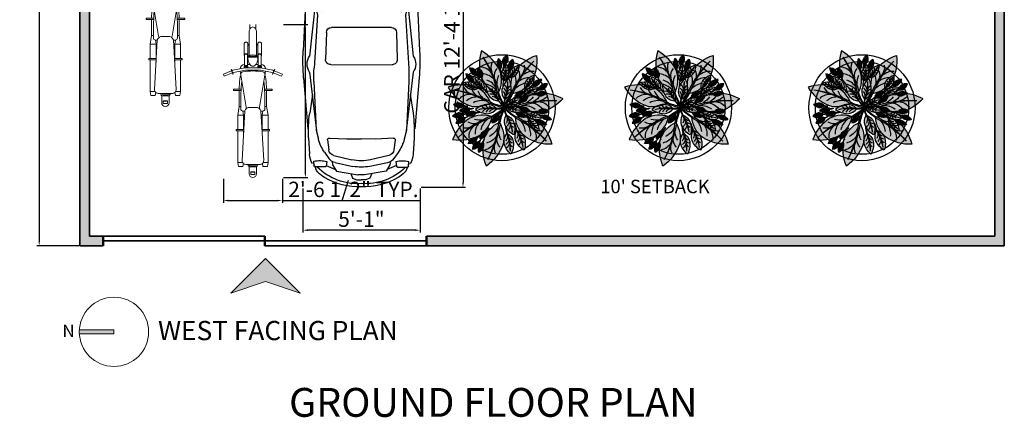
# Model space of a CAD drawing. Units: inches. Extents: x 3008 to 4088, y 1255 to 2137.
# Tile 1 of 30: x 3008 to 3520, y 1255 to 1462. Entities that reach past the tile are written whole.
import ezdxf

# ---------------------------------------------------------------- set-up
doc = ezdxf.new("R2010")
doc.units = ezdxf.units.IN
for name, color, linetype, lineweight in [('A-ANNO-DIMS', 2, 'Continuous', 18), ('A-ANNO-SYMB', 7, 'Continuous', 18), ('A-ANNO-TEXT', 7, 'Continuous', 18), ('A-WALL', 7, 'Continuous', 50), ('C-PROP', 1, 'Continuous', 35), ('C-PROP-PATT', 9, 'Continuous', 13), ('C-SITE-VEHC', 9, 'Continuous', 13), ('L-PLNT', 3, 'Continuous', 13)]:
    doc.layers.add(name, color=color, linetype=linetype, lineweight=lineweight)
doc.layers.add('L9012X$0', color=2, linetype='Continuous')
doc.layers.add('MESA', color=7, linetype='Continuous')
doc.styles.get("Standard").update_dxf_attribs({"font": 'arial.ttf'})
doc.dimstyles.new('ISO-25', dxfattribs={"dimtxt": 8, "dimasz": 2.5, "dimexe": 1.25, "dimexo": 0.625, "dimtad": 1, "dimdec": 1, "dimlunit": 3, "dimtxsty": 'Standard', "dimcen": 2.5, "dimadec": 0, "dimazin": 0, "dimtfac": 1, "dimtdec": 1, "dimtmove": 0, "dimatfit": 3, "dimfxl": 1, "dimarcsym": 0})

# ---------------------------------------------------------------- blocks, each defined once
blk = doc.blocks.new('*D2')
at = {"layer": 'A-ANNO-DIMS', "color": 0, "lineweight": -2, "transparency": 16777216}
for p, q in [((3039.04, 2003.97), (3017.26, 2003.97)), ((3018.51, 2001.47), (3018.51, 1346.47)), ((3039.04, 1343.97), (3017.26, 1343.97))]:
    blk.add_line(p, q, dxfattribs=at)
at = {"layer": 'A-ANNO-DIMS', "color": 0, "transparency": 16777216}
for points in [[(3018.09, 2001.47), (3018.93, 2001.47), (3018.51, 2003.97)], [(3018.09, 1346.47), (3018.93, 1346.47), (3018.51, 1343.97)]]:
    blk.add_solid(points, dxfattribs=at)
at = {"layer": 'Defpoints', "color": 0, "transparency": 16777216}
for p in [(3039.67, 2003.97), (3018.51, 1343.97), (3039.67, 1343.97)]:
    blk.add_point(p, dxfattribs=at)
at = {"layer": 'A-ANNO-DIMS', "color": 0, "transparency": 16777216, "insert": (3013.82, 1673.97), "char_height": 8, "attachment_point": 5, "rotation": 90}
blk.add_mtext("55'", dxfattribs=at)
blk = doc.blocks.new('A1099DC')
at = {"color": 0, "linetype": 'ByBlock'}
for p, q in [((272.228253, 749.073842), (265.114727, 718.465169)), ((1279.298465, 804.448389), (2201.430588, 851.890505)), ((1475.52921, 670.226262), (2282.402739, 758.004075)), ((2519.280414, 756.817792), (3387.476361, 653.818028)), ((2602.736326, 846.078152), (3356.693814, 785.353187)), ((2851.341839, 715.213377), (3126.60716, 755.701993)), ((3488.458929, 772.663345), (3732.658862, 759.86454)), ((92.537504, 388.14361), (139.051458, 595.027331)), ((139.051458, 595.027331), (190.951238, 683.213377)), ((179.200345, 564.515703), (190.951238, 709.631982)), ((405.405047, 577.538958), (396.874865, 615.894428)), ((398.733388, 644.315148), (411.280494, 678.748261)), ((589.014326, 626.599587), (405.405047, 577.538958)), ((411.280494, 678.748261), (588.616917, 641.417897)), ((1482.852352, 674.283145), (1175.286956, 622.180789)), ((1300.814287, 466.658131), (1445.712032, 613.104998)), ((1465.665584, 620.56924), (1602.893878, 610.287296)), ((1494.603245, 682.841284), (1678.210958, 641.166865)), ((1626.354615, 583.507504), (1602.652901, 169.222264)), ((1678.210958, 641.166865), (2462.684993, 690.847736)), ((2656.476214, 692.831247), (3376.704709, 662.004075)), ((3376.704709, 662.004075), (3510.708679, 626.736433)), ((3909.27561, 688.812956), (3837.725727, 693.401722)), ((3867.794139, 700.329656), (3900.059395, 686.767505)), ((3921.162781, 527.618662), (3921.162781, 676.138994)), ((3925.383812, 676.122818), (3955.306409, 663.545364)), ((236.043912, 551.980927), (179.200345, 564.515703)), ((229.117398, 477.634662), (225.714299, 427.957563)), ((1933.148906, 509.557888), (2330.980062, 522.200075)), ((2409.60024, 445.938054), (2410.49349, -460.09121)), ((3493.960271, 465.734554), (3507.923021, 209.166865)), ((3522.252709, 492.345257), (3666.066199, 475.644444)), ((3704.596898, 536.993674), (3795.675135, 473.385795)), ((3841.786866, 503.451367), (3910.58243, 515.096797)), ((3901.001848, 514.780764), (3957.150905, 375.772812)), ((57.774444, 216.608726), (92.537504, 388.14361)), ((1235.045743, 136.116317), (1257.419842, 373.755108)), ((1860.238743, -448.635916), (1859.369151, 433.397797)), ((3753.293176, 397.789551), (3815.226005, 132.124765)), ((3839.396146, 426.841284), (3888.358202, 417.538958)), ((3857.610793, 379.525702), (3912.067615, 118.157673)), ((3888.358202, 417.538958), (3983.199613, 359.957848)), ((3983.199613, 359.957848), (4035.448301, 43.94997)), ((49.168662, 58.00681), (57.774444, 216.608726)), ((3507.923021, 209.166865), (3507.64153, -4.333678)), ((4019.086894, 150.376168), (4084.69605, 122.469191)), ((4084.69605, 122.469191), (4109.177079, 60.329656)), ((4109.177079, 60.329656), (4113.094043, -5.158716)), ((49.301278, -76.507426), (58.219773, -235.092064)), ((3508.347273, -221.154823), (3507.644805, -7.65525)), ((3754.088875, -409.293325), (3815.497749, -143.506937)), ((3858.370276, -390.823819), (3912.311631, -129.348921)), ((3983.920268, -371.008369), (4035.545755, -54.898082)), ((4019.394229, -161.356334), (4084.948231, -133.320044)), ((4084.948231, -133.320044), (4109.306686, -71.132359)), ((4109.306686, -71.132359), (4113.094514, -5.636391)), ((58.219773, -235.092064), (93.320996, -406.558069)), ((1235.330373, -152.586046), (1258.173002, -390.180259)), ((1627.520644, -599.204785), (1603.002095, -184.967086)), ((3494.890446, -477.749545), (3508.347273, -221.154823)), ((93.320996, -406.558069), (140.24279, -613.349673)), ((3840.248961, -438.175225), (3889.19258, -428.776374)), ((3889.19258, -428.776374), (3983.920268, -371.008369)), ((3902.027941, -525.993061), (3957.902795, -386.874665)), ((237.150178, -570.112104), (180.331436, -582.758939)), ((230.077082, -495.779641), (226.576036, -446.109349)), ((1301.750547, -482.997536), (1446.936772, -629.158411)), ((1934.168526, -524.650381), (2332.023837, -536.508105)), ((3523.2353, -504.304409), (3667.01558, -487.320059)), ((3705.667171, -548.593196), (3796.61981, -484.805853)), ((3842.790735, -514.780444), (3911.609128, -526.290202)), ((3922.214148, -538.79118), (3922.506998, -687.311224)), ((140.24279, -613.349673), (192.316354, -701.433212)), ((180.331436, -582.758939), (192.368445, -727.851766)), ((406.561378, -595.336142), (398.106841, -633.708356)), ((400.0214, -662.125356), (412.636377, -696.533662)), ((590.267037, -644.034637), (406.561378, -595.336142)), ((412.636377, -696.533662), (589.898847, -658.853701)), ((1484.19765, -690.263206), (1176.530118, -638.767405)), ((1466.905004, -636.583294), (1604.112757, -626.030785)), ((1476.866524, -686.22077), (2283.911563, -772.40743)), ((1495.965396, -698.798158), (1679.490579, -656.761786)), ((1679.490579, -656.761786), (2464.061049, -704.895745)), ((2520.786439, -770.754078), (3388.777604, -666.042617)), ((2657.855804, -706.497136), (3378.022114, -674.249887)), ((3378.022114, -674.249887), (3511.956283, -638.718087)), ((3910.644841, -700.0086), (3839.104145, -704.738438)), ((3869.186159, -711.60707), (3901.424611, -697.981326)), ((3926.727989, -687.286725), (3956.625729, -674.650294)), ((273.723073, -767.133288), (266.549207, -736.538701)), ((1280.900818, -820.829563), (2203.124693, -866.453338)), ((2604.418191, -859.849707), (3358.254477, -797.638217)), ((2852.765183, -728.494989), (3128.109803, -768.440762)), ((3489.994314, -784.688586), (3734.168535, -771.408296))]:
    blk.add_line(p, q, dxfattribs=at)
for points in [[(-0.000783, 0.794772), (5.385043, 172.701749), (63.649891, 493.818028), (92.537504, 603.957563), (144.437284, 705.166865), (428.417214, 824.236633), (585.095796, 846.190121), (961.406447, 846.190121), (1274.27399, 797.818028), (1482.852352, 709.631982)], [(83.345007, -3.206171), (111.32237, 268.957533), (164.563706, 379.583828), (279.999271, 453.709838), (456.549665, 511.628518), (901.254996, 574.918954), (1175.286956, 622.180789), (1137.52997, 385.548359), (1118.345181, 137.317882), (1109.829198, -8.358455)], [(168.178729, 359.003083), (1030.214866, 528.397865), (1077.798844, 510.531569), (1086.170082, 475.285426), (992.832238, 91.960378), (924.218938, 35.478085), (108.447994, 6.034416)], [(0.019119, -19.392451), (5.743899, -191.288474), (64.641806, -512.289243), (93.746535, -622.371603), (145.845778, -723.478374), (430.059935, -841.987962), (586.7815, -863.632471), (963.091723, -863.198028), (1275.863278, -814.209121), (1484.26735, -725.611974)], [(83.356858, -15.227176), (111.870816, -287.335185), (165.330179, -397.856284), (280.911681, -471.754535), (457.575935, -529.324983), (902.4055, -592.045995), (1176.530118, -638.767405), (1138.306616, -402.209884), (1118.632407, -154.017717), (1109.829198, -8.358455)], [(168.904615, -377.268451), (1031.273389, -545.270714), (1078.822046, -527.310627), (1087.123771, -492.048047), (993.030273, -108.907787), (924.305735, -52.560894), (108.478017, -24.418246)]]:
    blk.add_lwpolyline(points, dxfattribs=at)
for centre, radius, start, end in [((2358.037832, -2192.08357), 3048, 85.395244, 92.945173), ((2399.99649, 588.663508), 206.166238, 54.649181, 124.776949), ((3392.740754, -1053.630025), 1828.8, 86.999806, 98.367602), ((3718.678317, 475.802507), 284.405862, 57.329946, 87.182375), ((1749.553982, 373.478072), 1524, 166.916578, 176.08111), ((446.46332, 626.922805), 50.8, 159.97873, 192.538409), ((587.047263, 633.961317), 7.62, 284.960009, 78.112462), ((1463.767788, 595.240237), 25.4, 85.715073, 135.304647), ((1600.996082, 584.958293), 25.4, 356.725615, 85.715073), ((2578.271641, -1134.295865), 1828.8, 87.549126, 93.623712), ((3355.555414, 37.211519), 609.6, 55.070043, 75.255062), ((4191.049821, 605.937201), 363.988953, 166.096081, 196.353514), ((3908.462781, 676.138994), 12.7, 0, 86.330429), ((3320.85101, 50.338397), 847.430844, 356.245089, 44.519453), ((3896.252417, 523.051998), 152.4, 46.38363, 67.20138), ((3700.933354, 318.064082), 435.542335, 30.457681, 46.38363), ((1409.148822, 359.469565), 152.4, 135.304647, 174.62136), ((1935.569151, 433.396333), 76.2, 91.82012, 179.9989), ((2333.400307, 446.03852), 76.2, 359.924458, 91.82012), ((3519.322741, 467.114813), 25.4, 83.37601, 183.115039), ((3654.346327, 374.722669), 101.6, 13.122645, 83.37601), ((3708.414764, 348.440256), 152.4, 11.769371, 55.070043), ((3908.462781, 527.618662), 12.7, 279.607718, 0), ((3204.184594, 25.950693), 1011.814461, 358.069446, 30.457681), ((4645.676894, -4.872483), 3048, 176.725615, 183.38736), ((1266.577845, -8.050136), 1219.2, 176.894161, 183.218814), ((2752.335538, -6.739118), 1524, 174.62136, 185.491615), ((3221.54491, -6.276527), 609.6, 346.99033, 13.122645), ((3315.283499, -6.18411), 609.6, 348.343604, 11.769371), ((3734.73098, -5.770579), 304.8, 350.724636, 9.388339), ((3320.962449, -62.69553), 847.430844, 315.593523, 3.867886), ((3204.248172, -38.537915), 1011.814461, 329.655294, 2.043529), ((1409.873518, -375.595566), 152.4, 185.491615, 224.808328), ((3655.096735, -386.42159), 101.6, 276.736965, 346.99033), ((3709.113243, -360.032616), 152.4, 305.042932, 348.343604), ((1750.305335, -388.625277), 1524, 184.031865, 193.196397), ((1936.438592, -448.484202), 76.2, 180.114076, 268.292856), ((2334.293902, -460.341926), 76.2, 268.292856, 0.188517), ((3520.255588, -479.079792), 25.4, 176.997936, 276.736965), ((3355.640902, -49.500248), 609.6, 284.857913, 305.042932), ((4192.255091, -616.577407), 363.988953, 163.759461, 194.016894), ((3909.514173, -538.816222), 12.7, 0.112975, 80.505257), ((3701.571953, -329.671253), 435.542335, 313.729345, 329.655294), ((447.716945, -644.638934), 50.8, 167.574566, 200.134245), ((588.314493, -651.400231), 7.62, 282.000513, 75.152966), ((1464.957267, -611.258083), 25.4, 224.808328, 274.397903), ((1602.165021, -600.705574), 25.4, 274.397903, 3.38736), ((2576.048678, 1120.472221), 1828.8, 266.489263, 272.563849), ((3719.627907, -487.374382), 284.405862, 272.930601, 302.78303), ((3909.807023, -687.336265), 12.7, 273.782546, 0.112975), ((3897.294828, -534.273643), 152.4, 292.911596, 313.729345), ((2353.729565, 2177.823616), 3048, 267.167802, 274.717731), ((2401.171182, -602.835323), 206.166238, 235.336026, 305.463794), ((3390.675263, 1041.412497), 1828.8, 261.745373, 273.113169)]:
    blk.add_arc(centre, radius, start, end, dxfattribs=at)
blk = doc.blocks.new('VI')
at = {"layer": 'L9012X$0'}
blk.add_blockref('A1099DC', (0, 0), dxfattribs=at)
blk = doc.blocks.new('BIKE')
for p, q in [((34846.04, 15170.34), (34846.04, 15168.87)), ((34847.86, 15170.34), (34847.86, 15168.87)), ((34845.81, 15167.86), (34845.81, 15160.7)), ((34845.81, 15167.86), (34845.81, 15160.7)), ((34848.09, 15167.86), (34848.09, 15160.7)), ((34844.29, 15164.4), (34844.29, 15160.81)), ((34845.43, 15164.4), (34845.43, 15160.81)), ((34845.43, 15164.1), (34845.81, 15164.1)), ((34845.43, 15163.85), (34845.81, 15163.85)), ((34848.47, 15164.1), (34848.09, 15164.1)), ((34848.47, 15163.85), (34848.09, 15163.85)), ((34848.47, 15164.4), (34848.47, 15160.81)), ((34849.61, 15164.4), (34849.61, 15160.81)), ((34844.41, 15160.81), (34844.41, 15157.43)), ((34845.32, 15160.81), (34845.32, 15157.43)), ((34848.51, 15160.53), (34845.39, 15160.53)), ((34845.39, 15160.23), (34845.39, 15160.53)), ((34845.39, 15160.23), (34845.39, 15160.53)), ((34848.51, 15160.23), (34848.51, 15160.53)), ((34848.58, 15160.81), (34848.58, 15157.43)), ((34849.5, 15160.81), (34849.5, 15157.43)), ((34845.32, 15157.92), (34846.04, 15157.92)), ((34848.51, 15160.23), (34845.39, 15160.23)), ((34848.58, 15157.92), (34847.87, 15157.92)), ((34837.84, 15154.89), (34840.37, 15155.93)), ((34837.84, 15154.89), (34838.1, 15154.26)), ((34838.1, 15154.26), (34840.63, 15155.3)), ((34840.19, 15156.35), (34840.3, 15156.39)), ((34840.19, 15156.35), (34840.8, 15154.88)), ((34840.3, 15156.39), (34840.9, 15154.92)), ((34840.47, 15155.97), (34840.8, 15156.11)), ((34840.73, 15155.34), (34841, 15155.45)), ((34840.8, 15156.11), (34844.56, 15156.88)), ((34840.8, 15154.88), (34840.9, 15154.92)), ((34841, 15155.45), (34844.63, 15156.2)), ((34842.8, 15152.59), (34843.06, 15154.2)), ((34844.86, 15144.72), (34843.01, 15155.87)), ((34843.06, 15154.2), (34843.22, 15154.58)), ((34844.29, 15156.87), (34844.29, 15157.17)), ((34844.41, 15156.87), (34844.41, 15156.85)), ((34844.56, 15156.88), (34846.95, 15156.88)), ((34844.63, 15156.2), (34846.95, 15156.2)), ((34845.43, 15156.87), (34845.43, 15157.17)), ((34849.34, 15156.88), (34846.95, 15156.88)), ((34849.27, 15156.2), (34846.95, 15156.2)), ((34848.47, 15156.87), (34848.47, 15157.17)), ((34849.05, 15144.72), (34850.89, 15155.87)), ((34852.9, 15155.45), (34849.27, 15156.2)), ((34853.1, 15156.11), (34849.34, 15156.88)), ((34849.5, 15156.87), (34849.5, 15156.85)), ((34849.61, 15156.87), (34849.61, 15157.17)), ((34850.84, 15154.2), (34850.68, 15154.58)), ((34851.1, 15152.59), (34850.84, 15154.2)), ((34853.17, 15155.34), (34852.9, 15155.45)), ((34853.6, 15156.39), (34853, 15154.92)), ((34853.1, 15154.88), (34853, 15154.92)), ((34853.71, 15156.35), (34853.1, 15154.88)), ((34853.43, 15155.97), (34853.1, 15156.11)), ((34855.81, 15154.26), (34853.28, 15155.3)), ((34856.07, 15154.89), (34853.54, 15155.93)), ((34853.71, 15156.35), (34853.6, 15156.39)), ((34856.07, 15154.89), (34855.81, 15154.26)), ((34842.7, 15150.31), (34842.8, 15152.59)), ((34843.33, 15151.09), (34843.52, 15152.8)), ((34850.57, 15151.09), (34850.38, 15152.8)), ((34851.2, 15150.31), (34851.1, 15152.59)), ((34840.97, 15150.31), (34843.3, 15150.31)), ((34840.97, 15149.81), (34840.97, 15150.31)), ((34843.29, 15149.81), (34840.97, 15149.81)), ((34842.7, 15144.87), (34842.7, 15149.81)), ((34843.23, 15147.75), (34843.33, 15151.09)), ((34850.67, 15147.75), (34850.57, 15151.09)), ((34852.93, 15150.31), (34850.6, 15150.31)), ((34850.61, 15149.81), (34852.93, 15149.81)), ((34851.2, 15144.87), (34851.2, 15149.81)), ((34852.93, 15149.81), (34852.93, 15150.31)), ((34843.23, 15144.15), (34843.23, 15147.75)), ((34850.67, 15144.15), (34850.67, 15147.75)), ((34842.7, 15144.87), (34842.25, 15142.19)), ((34842.25, 15142.19), (34844.07, 15142.19)), ((34842.25, 15137.82), (34842.25, 15142.19)), ((34842.7, 15144.87), (34843.23, 15144.87)), ((34844.46, 15143.56), (34843.6, 15128.2)), ((34843.85, 15143.46), (34844.07, 15142.19)), ((34843.91, 15143.46), (34844.46, 15143.46)), ((34844.07, 15137.82), (34844.07, 15142.19)), ((34847.85, 15144.64), (34846.06, 15144.64)), ((34849.44, 15143.56), (34850.3, 15128.2)), ((34849.99, 15143.46), (34849.44, 15143.46)), ((34850.05, 15143.46), (34849.83, 15142.19)), ((34851.65, 15142.19), (34849.83, 15142.19)), ((34849.83, 15137.82), (34849.83, 15142.19)), ((34851.2, 15144.87), (34850.67, 15144.87)), ((34851.2, 15144.87), (34851.65, 15142.19)), ((34851.65, 15137.82), (34851.65, 15142.19)), ((34841.79, 15137.82), (34844.14, 15137.82)), ((34841.79, 15137.33), (34841.79, 15137.82)), ((34844.11, 15137.33), (34841.79, 15137.33)), ((34842.25, 15127.57), (34842.25, 15137.33)), ((34844.07, 15136.55), (34844.07, 15137.33)), ((34852.11, 15137.82), (34849.76, 15137.82)), ((34849.79, 15137.33), (34852.11, 15137.33)), ((34849.83, 15136.55), (34849.83, 15137.33)), ((34851.65, 15127.57), (34851.65, 15137.33)), ((34852.11, 15137.33), (34852.11, 15137.82)), ((34842.25, 15127.57), (34843.75, 15127.57)), ((34842.25, 15127.57), (34842.48, 15126.27)), ((34844.02, 15127.25), (34843.84, 15126.27)), ((34849.16, 15126.99), (34844.74, 15126.99)), ((34845.47, 15126.99), (34845.47, 15126.88)), ((34845.81, 15126.99), (34845.81, 15126.88)), ((34848.09, 15126.99), (34848.09, 15126.88)), ((34848.43, 15126.99), (34848.43, 15126.88)), ((34849.89, 15127.25), (34850.06, 15126.27)), ((34851.65, 15127.57), (34850.15, 15127.57)), ((34851.65, 15127.57), (34851.43, 15126.27)), ((34842.48, 15126.27), (34843.84, 15126.27)), ((34845.81, 15126.29), (34845.81, 15124.03)), ((34847.75, 15126.54), (34846.15, 15126.54)), ((34847.75, 15126.2), (34846.15, 15126.2)), ((34846.29, 15123.82), (34846.29, 15124.66)), ((34846.29, 15124.66), (34847.61, 15124.66)), ((34846.29, 15124.55), (34847.61, 15124.55)), ((34847.61, 15123.82), (34846.29, 15123.82)), ((34847.61, 15124.66), (34847.61, 15123.82)), ((34848.09, 15126.29), (34848.09, 15124.03)), ((34851.43, 15126.27), (34850.06, 15126.27))]:
    blk.add_line(p, q)
for points in [[(34845.81, 15167.86, -0.068977), (34845.9, 15168.53, -0.081012), (34846.15, 15169.05, -0.107014), (34846.54, 15169.42, -0.137239), (34846.95, 15169.53, -0.137239), (34847.36, 15169.42, -0.107014), (34847.76, 15169.05, -0.081012), (34848, 15168.53, -0.068977), (34848.09, 15167.86, -0.068977)], [(34845.43, 15164.4, 0.125099), (34845.39, 15164.56, 0.105827), (34845.27, 15164.71, 0.086577), (34845.09, 15164.8, 0.0766), (34844.86, 15164.84, 0.0766), (34844.64, 15164.8, 0.086577), (34844.46, 15164.71, 0.105827), (34844.33, 15164.56, 0.125099), (34844.29, 15164.4, 0.125099)], [(34848.47, 15164.4, -0.125099), (34848.51, 15164.56, -0.105827), (34848.64, 15164.71, -0.086577), (34848.82, 15164.8, -0.0766), (34849.04, 15164.84, -0.0766), (34849.26, 15164.8, -0.086577), (34849.44, 15164.71, -0.105827), (34849.57, 15164.56, -0.125099), (34849.61, 15164.4, -0.125099)], [(34845.32, 15160.55, 0.067261), (34845.39, 15160.65, 0.125099), (34845.43, 15160.81, 0.125099), (34845.39, 15160.97, 0.105827), (34845.27, 15161.12, 0.086577), (34845.09, 15161.21, 0.0766), (34844.86, 15161.25, 0.0766), (34844.64, 15161.21, 0.086577), (34844.46, 15161.12, 0.105827), (34844.33, 15160.97, 0.125099), (34844.29, 15160.81, 0.125099)], [(34844.29, 15160.81, 0.125099), (34844.33, 15160.65, 0.067261), (34844.41, 15160.55, 0.086577)], [(34845.32, 15160.81, 0.125099), (34845.29, 15160.92, 0.105827), (34845.2, 15161.03, 0.086577), (34845.05, 15161.1, 0.0766), (34844.86, 15161.13, 0.0766), (34844.67, 15161.1, 0.086577), (34844.53, 15161.03, 0.105827), (34844.43, 15160.92, 0.125099), (34844.41, 15160.81, 0.125099)], [(34848.58, 15160.55, -0.067261), (34848.51, 15160.65, -0.125099), (34848.47, 15160.81, -0.125099), (34848.51, 15160.97, -0.105827), (34848.64, 15161.12, -0.086577), (34848.82, 15161.21, -0.0766), (34849.04, 15161.25, -0.0766), (34849.26, 15161.21, -0.086577), (34849.44, 15161.12, -0.105827), (34849.57, 15160.97, -0.125099), (34849.61, 15160.81, -0.125099)], [(34848.58, 15160.81, -0.125099), (34848.61, 15160.92, -0.105827), (34848.71, 15161.03, -0.086577), (34848.85, 15161.1, -0.0766), (34849.04, 15161.13, -0.0766), (34849.23, 15161.1, -0.086577), (34849.37, 15161.03, -0.105827), (34849.47, 15160.92, -0.125099), (34849.5, 15160.81, -0.125099)], [(34849.61, 15160.81, -0.125099), (34849.57, 15160.65, -0.067261), (34849.5, 15160.55, -0.086577)], [(34845.43, 15157.17, 0.125099), (34845.39, 15157.33, 0.105827), (34845.27, 15157.48, 0.086577), (34845.09, 15157.57, 0.0766), (34844.86, 15157.6, 0.0766), (34844.64, 15157.57, 0.086577), (34844.46, 15157.48, 0.105827), (34844.33, 15157.33, 0.125099), (34844.29, 15157.17, 0.125099)], [(34845.43, 15156.88, 0.117252), (34845.39, 15157.03, 0.105827), (34845.27, 15157.18, 0.086577), (34845.09, 15157.27, 0.0766), (34844.86, 15157.31, 0.0766), (34844.64, 15157.27, 0.086577), (34844.46, 15157.18, 0.105827), (34844.33, 15157.03, 0.125099), (34844.29, 15156.87, 0.125099)], [(34846.95, 15157.37, -0.163989), (34846.41, 15157.55, -0.105862), (34845.85, 15158.21, -0.069323), (34845.52, 15159.08, -0.055531), (34845.39, 15160.23, -0.055531)], [(34848.51, 15160.23, -0.055531), (34848.38, 15159.08, -0.069323), (34848.06, 15158.21, -0.105862), (34847.49, 15157.55, -0.163989), (34846.95, 15157.37, -0.163989)], [(34848.47, 15157.17, -0.125099), (34848.51, 15157.33, -0.105827), (34848.64, 15157.48, -0.086577), (34848.82, 15157.57, -0.0766), (34849.04, 15157.6, -0.0766), (34849.26, 15157.57, -0.086577), (34849.44, 15157.48, -0.105827), (34849.57, 15157.33, -0.125099), (34849.61, 15157.17, -0.125099)], [(34848.47, 15156.88, -0.117252), (34848.51, 15157.03, -0.105827), (34848.64, 15157.18, -0.086577), (34848.82, 15157.27, -0.0766), (34849.04, 15157.31, -0.0766), (34849.26, 15157.27, -0.086577), (34849.44, 15157.18, -0.105827), (34849.57, 15157.03, -0.125099), (34849.61, 15156.87, -0.125099)], [(34844.29, 15156.87, 0.032819), (34844.3, 15156.83, 0.067261)], [(34845.32, 15156.88, 0.113202), (34845.29, 15156.98, 0.105827), (34845.2, 15157.09, 0.086577), (34845.05, 15157.16, 0.0766), (34844.86, 15157.19, 0.0766), (34844.67, 15157.16, 0.086577), (34844.53, 15157.09, 0.105827), (34844.43, 15156.98, 0.125099), (34844.41, 15156.87, 0.125099)], [(34848.58, 15156.88, -0.113202), (34848.61, 15156.98, -0.105827), (34848.71, 15157.09, -0.086577), (34848.85, 15157.16, -0.0766), (34849.04, 15157.19, -0.0766), (34849.23, 15157.16, -0.086577), (34849.37, 15157.09, -0.105827), (34849.47, 15156.98, -0.125099), (34849.5, 15156.87, -0.125099)], [(34849.61, 15156.87, -0.032819), (34849.61, 15156.83, -0.067261)]]:
    blk.add_lwpolyline(points, format="xyb")
for centre, radius, start, end in [((34846.95, 15157.24), 3.64, 64.5882, 115.4118), ((34844.55, 15156.32), 1.59, 95.2207, 171.678), ((34849.35, 15156.32), 1.59, 8.322, 84.7793), ((34843.86, 15154.92), 0.684, 90, 189.3898), ((34846.95, 15140.12), 15.79, 78.7129, 101.2871), ((34850.04, 15154.92), 0.684, 350.6102, 90), ((34843.91, 15144.15), 0.684, 180, 270), ((34846, 15143), 1.64, 88.1125, 159.9264), ((34845.53, 15144.83), 0.684, 189.3898, 226.4877), ((34847.9, 15143), 1.64, 20.0736, 91.8875), ((34848.37, 15144.83), 0.684, 313.5123, 350.6102), ((34849.99, 15144.15), 0.684, 270, 0), ((34844.74, 15128.13), 1.14, 176.7865, 270), ((34846.15, 15126.88), 0.684, 180, 270), ((34846.15, 15126.88), 0.342, 180, 270), ((34847.75, 15126.88), 0.684, 270, 0), ((34847.75, 15126.88), 0.342, 270, 0), ((34849.16, 15128.13), 1.14, 270, 3.2135), ((34846.95, 15124.03), 1.14, 180, 0)]:
    blk.add_arc(centre, radius, start, end)
blk = doc.blocks.new('folha Ant')
at = {"layer": 'MESA', "ltscale": 0.8}
h = blk.add_hatch(color=256, dxfattribs=at)
h.dxf.hatch_style = 1
h.set_gradient(color1=(103, 159, 96), color2=(179, 207, 175), one_color=1, tint=0.75, name='INVCURVED')
h.paths.add_polyline_path([(0.2266, 0.0676, 0.199512), (0.0989, 0.0067, 0.09675), (0.3533, 0.0075, -0.086654), (0.1023, -0.0053, 0.192489), (0.2266, -0.0624, 0.158608), (0.3953, 0.0026, 0.158608)])
h = blk.add_hatch(color=256, dxfattribs=at)
h.dxf.hatch_style = 1
h.set_gradient(color1=(179, 116, 77), color2=(114, 74, 49), one_color=1, tint=0.32, name='CURVED')
h.paths.add_polyline_path([(0.05, -0.0003), (0.0485, 0.0057, 0.033108), (0, 0, 0.809082), (0.002, -0.006, -0.032777)])
h.paths.add_polyline_path([(0.0973, 0.0049, 0.033108), (0.0485, 0.0057), (0.05, -0.0003, -0.032777), (0.0983, -0.001), (0.0953, 0.0026)])
h = blk.add_hatch(color=256, dxfattribs=at)
h.dxf.hatch_style = 1
h.set_gradient(color1=(103, 159, 96), color2=(52, 80, 48), one_color=1, tint=0.25)
h.paths.add_polyline_path([(0.3533, 0.0075, -0.09675), (0.0989, 0.0067, 0.007527), (0.0953, 0.0026, 0.014292), (0.1023, -0.0053, 0.086654)])
blk.add_lwpolyline([(0.0983, -0.001), (0.0953, 0.0026), (0.0973, 0.0049, 0.066288), (0, 0, 0.809082), (0.002, -0.006, -0.065625)], format="xyb", close=True, dxfattribs=at)
for centre, radius, start, end in [((0.2359, -0.1164), 0.1842, 92.91214, 139.76953), ((0.211, -0.2242), 0.2922, 50.90546, 86.95539), ((0.2359, 0.1215), 0.1842, 220.23047, 267.08786), ((0.2242, 0.6583), 0.6635, 259.11898, 281.22354), ((0.1912, 0.7199), 0.7306, 263.00966, 282.81986), ((0.1144, 0.1192), 0.1187, 277.64114, 318.48201), ((0.1515, 0.1013), 0.1129, 290.56342, 330.45391), ((0.211, 0.2293), 0.2922, 273.04461, 309.09454), ((0.2123, 0.0879), 0.0955, 283.00127, 333.19107), ((0.1127, -0.1239), 0.1214, 41.75279, 70.10606), ((0.1853, -0.0821), 0.0727, 27.73756, 79.23475), ((0.2381, -0.0995), 0.0902, 48.80268, 88.01103)]:
    blk.add_arc(centre, radius, start, end, dxfattribs=at)
blk = doc.blocks.new('arvore L')
at = {"layer": 'MESA', "ltscale": 0.8}
for radius in [0.35, 0.3077]:
    blk.add_circle((-0.0174, -0.0123), radius, dxfattribs=at)
at = {"layer": 'MESA'}
for p, rotation in [((-0.0038, -0.0034), 111.8634939329907), ((-0.0015, -0.0116), 159.7023978146411), ((-0.002, -0.0223), 210.0932896211622)]:
    blk.add_blockref('folha Ant', p, dxfattribs=dict(at, rotation=rotation))
at = {"layer": 'MESA', "xscale": -1}
for p, rotation in [((-0.0038, 0.0015), 237.4553048776787), ((-0.0054, -0.0158), 189.5771815307885), ((-0.0065, -0.0187), 73.74235818062448), ((-0.0036, -0.0152), 143.2116612097536)]:
    blk.add_blockref('folha Ant', p, dxfattribs=dict(at, rotation=rotation))
at = {"layer": 'MESA'}
for p, xscale, yscale, zscale, rotation in [((-0.0106, 0.2458), -0.2372171158460138, 0.2372171158460219, 0.2372171158460401, 254.670727296299), ((-0.1648, 0.1856), 0.2372171158460308, 0.2372171158460308, 0.2372171158460308, 134.9461414081513), ((-0.0228, 0.2207), 0.2372171158460145, 0.2372171158460145, 0.2372171158460145, 100.7442899234288), ((-0.0127, 0.1293), 0.367298872610303, 0.367298872610303, 0.367298872610303, 78.9591877781593), ((0.0048, 0.1582), 0.3672988726102984, 0.3672988726102984, 0.3672988726102984, 49.45009658216958), ((0.0276, 0.2187), -0.2372171158460138, 0.2372171158460219, 0.2372171158460401, 254.670727296299), ((-0.189, 0.1454), 0.2372171158460308, 0.2372171158460308, 0.2372171158460308, 134.9461414081513), ((-0.1144, 0.0854), -0.3672988726103342, 0.3672988726103199, 0.3672988726103326, 310.6576809262878), ((-0.1441, 0.1612), -0.2372171158460326, 0.2372171158460219, 0.2372171158460401, 288.8725787810177), ((0.1186, 0.0777), -0.3672988726103297, 0.3672988726103199, 0.3672988726103326, 240.0025576387842), ((-0.1408, 0.1026), -0.3672988726103232, 0.3672988726103199, 0.3672988726103326, 340.1667721222815), ((-0.0091, -0.003), 0.4722192998870449, 0.4722192998870449, 0.4722192998870449, 127.7597565182155), ((-0.0068, -0.0029), 0.4722192998870434, 0.4722192998870434, 0.4722192998870434, 78.95918777814883), ((0.0972, 0.0516), -0.3672988726102771, 0.3672988726103199, 0.3672988726103326, 210.4934664427891), ((0.1681, 0.1193), 0.2372171158460773, 0.2372171158460773, 0.2372171158460773, 34.78192692463861), ((0.2063, 0.0923), 0.2372171158460773, 0.2372171158460773, 0.2372171158460773, 34.78192692463861), ((-0.0206, -0.0213), -0.3672988726102771, 0.3672988726103199, 0.3672988726103326, 210.4934664427891), ((0.0473, 0.041), 0.2372171158460773, 0.2372171158460773, 0.2372171158460773, 34.78192692463861), ((0.0807, 0.0116), 0.2372171158460773, 0.2372171158460773, 0.2372171158460773, 34.78192692463861), ((0.1867, 0.0725), -0.237217115846069, 0.2372171158460219, 0.2372171158460401, 188.7083642975024), ((-0.2438, -0.0026), 0.2372171158460885, 0.2372171158460885, 0.2372171158460885, 173.1881796188063), ((-0.0061, -0.0164), 0.4722192998870134, 0.4722192998870134, 0.4722192998870134, 181.8145453364702), ((-0.0239, 0.0106), 0.3672988726102808, 0.3672988726102808, 0.3672988726102808, 341.2516722292817), ((0.082, -0.001), -0.2372171158460231, 0.2372171158460219, 0.2372171158460401, 156.9632117474216), ((-0.2506, -0.0512), 0.2372171158460153, 0.2372171158460153, 0.2372171158460153, 190.4360105724469), ((-0.241, -0.0679), 0.237217115846034, 0.237217115846034, 0.237217115846034, 209.7732768087273), ((-0.2046, -0.0159), 0.2372171158460153, 0.2372171158460153, 0.2372171158460153, 190.4360105724469), ((-0.1644, -0.0415), 0.2372171158460153, 0.2372171158460153, 0.2372171158460153, 190.4360105724469), ((-0.024, -0.0418), -0.2372171158460388, 0.2372171158460219, 0.2372171158460401, 51.68033384933957), ((-0.0047, -0.0173), -0.4722192998870682, 0.4722192998870583, 0.4722192998870367, 110.7618316866296), ((0.0552, -0.0366), -0.2372171158460231, 0.2372171158460219, 0.2372171158460401, 156.9632117474216), ((0.1063, -0.0368), 0.3672988726102808, 0.3672988726102808, 0.3672988726102808, 341.2516722292817), ((0.1326, -0.058), 0.3672988726103005, 0.3672988726103005, 0.3672988726103005, 311.7425810332929), ((0.1982, -0.0391), 0.2372171158460078, 0.2372171158460078, 0.2372171158460078, 3.036774374557308), ((0.2214, -0.0544), -0.2372171158460231, 0.2372171158460219, 0.2372171158460401, 156.9632117474216), ((0.0082, -0.1357), -0.4722192998870255, 0.4722192998870583, 0.4722192998870367, 100.6603657106226), ((0.0645, -0.1182), -0.4722192998870682, 0.4722192998870583, 0.4722192998870367, 110.7618316866296), ((0.1895, -0.0887), -0.2372171158460231, 0.2372171158460219, 0.2372171158460401, 156.9632117474216), ((-0.1617, -0.1996), -0.2372171158460624, 0.2372171158460219, 0.2372171158460401, 32.34306761306672), ((-0.1025, -0.1443), -0.2372171158460388, 0.2372171158460219, 0.2372171158460401, 51.68033384933957), ((-0.1514, -0.2159), -0.2372171158460388, 0.2372171158460219, 0.2372171158460401, 51.68033384933957), ((-0.1351, -0.2206), -0.2372171158460438, 0.2372171158460219, 0.2372171158460401, 68.92816480300668)]:
    blk.add_blockref('folha Ant', p, dxfattribs=dict(at, xscale=xscale, yscale=yscale, zscale=zscale, rotation=rotation))
blk = doc.blocks.new('*D61')
at = {"layer": 'A-ANNO-DIMS', "color": 0, "lineweight": -2, "transparency": 16777216}
for p, q in [((3156.71, 1459.08), (3156.71, 1600.04)), ((3145.38, 1459.08), (3157.96, 1459.08)), ((3156.71, 1381.91), (3156.71, 1456.58)), ((3145.38, 1379.41), (3157.96, 1379.41))]:
    blk.add_line(p, q, dxfattribs=at)
at = {"layer": 'A-ANNO-DIMS', "color": 0, "transparency": 16777216}
for points in [[(3156.29, 1456.58), (3157.12, 1456.58), (3156.71, 1459.08)], [(3156.29, 1381.91), (3157.12, 1381.91), (3156.71, 1379.41)]]:
    blk.add_solid(points, dxfattribs=at)
at = {"layer": 'Defpoints', "color": 0, "transparency": 16777216}
for p in [(3144.76, 1459.08), (3156.71, 1459.08), (3144.76, 1379.41)]:
    blk.add_point(p, dxfattribs=at)
at = {"layer": 'A-ANNO-DIMS', "color": 0, "transparency": 16777216, "insert": (3151.94, 1530.81), "char_height": 8, "attachment_point": 5, "rotation": 90}
blk.add_mtext('MOTORBIKE 6\'-7 1/2" TYP.', dxfattribs=at)
blk = doc.blocks.new('*D62')
at = {"layer": 'A-ANNO-DIMS', "color": 0, "lineweight": -2, "transparency": 16777216}
for p, q in [((3114.15, 1378.79), (3114.15, 1366.21)), ((3144.76, 1378.79), (3144.76, 1366.21)), ((3116.65, 1367.46), (3142.26, 1367.46)), ((3144.76, 1367.46), (3216.05, 1367.46))]:
    blk.add_line(p, q, dxfattribs=at)
at = {"layer": 'A-ANNO-DIMS', "color": 0, "transparency": 16777216}
for points in [[(3116.65, 1367.88), (3116.65, 1367.05), (3114.15, 1367.46)], [(3142.26, 1367.88), (3142.26, 1367.05), (3144.76, 1367.46)]]:
    blk.add_solid(points, dxfattribs=at)
at = {"layer": 'Defpoints', "color": 0, "transparency": 16777216}
for p in [(3114.15, 1379.41), (3144.76, 1379.41), (3144.76, 1367.46)]:
    blk.add_point(p, dxfattribs=at)
at = {"layer": 'A-ANNO-DIMS', "color": 0, "transparency": 16777216, "insert": (3181.65, 1372.23), "char_height": 8, "attachment_point": 5}
blk.add_mtext('2\'-6 1/2" TYP.', dxfattribs=at)
blk = doc.blocks.new('*D63')
at = {"layer": 'A-ANNO-DIMS', "color": 0, "lineweight": -2, "transparency": 16777216}
for p, q in [((3216.92, 1522.92), (3239.83, 1522.92)), ((3238.58, 1520.42), (3238.58, 1376.84)), ((3216.92, 1374.34), (3239.83, 1374.34))]:
    blk.add_line(p, q, dxfattribs=at)
at = {"layer": 'A-ANNO-DIMS', "color": 0, "transparency": 16777216}
for points in [[(3238.16, 1520.42), (3238.99, 1520.42), (3238.58, 1522.92)], [(3238.16, 1376.84), (3238.99, 1376.84), (3238.58, 1374.34)]]:
    blk.add_solid(points, dxfattribs=at)
at = {"layer": 'Defpoints', "color": 0, "transparency": 16777216}
for p in [(3216.29, 1522.92), (3216.29, 1374.34), (3238.58, 1374.34)]:
    blk.add_point(p, dxfattribs=at)
at = {"layer": 'A-ANNO-DIMS', "color": 0, "transparency": 16777216, "insert": (3233.82, 1448.63), "char_height": 8, "attachment_point": 5, "rotation": 90}
blk.add_mtext('CAR 12\'-4 1/2"', dxfattribs=at)
blk = doc.blocks.new('*D64')
at = {"layer": 'A-ANNO-DIMS', "color": 0, "lineweight": -2, "transparency": 16777216}
for p, q in [((3155.35, 1373.71), (3155.35, 1350.8)), ((3216.29, 1373.71), (3216.29, 1350.8)), ((3213.79, 1352.05), (3157.85, 1352.05))]:
    blk.add_line(p, q, dxfattribs=at)
at = {"layer": 'A-ANNO-DIMS', "color": 0, "transparency": 16777216}
for points in [[(3157.85, 1352.47), (3157.85, 1351.63), (3155.35, 1352.05)], [(3213.79, 1352.47), (3213.79, 1351.63), (3216.29, 1352.05)]]:
    blk.add_solid(points, dxfattribs=at)
at = {"layer": 'Defpoints', "color": 0, "transparency": 16777216}
for p in [(3155.35, 1374.34), (3216.29, 1374.34), (3155.35, 1352.05)]:
    blk.add_point(p, dxfattribs=at)
at = {"layer": 'A-ANNO-DIMS', "color": 0, "transparency": 16777216, "insert": (3185.82, 1356.76), "char_height": 8, "attachment_point": 5}
blk.add_mtext('5\'-1"', dxfattribs=at)

msp = doc.modelspace()

# ---------------------------------------------------------------- hatches: boundary and pattern name
at = {"layer": 'A-ANNO-SYMB'}
h = msp.add_hatch(color=256, dxfattribs=at)
h.dxf.hatch_style = 1
h.paths.add_polyline_path([(3118, 1319.35), (3136, 1325.35), (3154, 1319.35), (3136, 1337.35)])
h = msp.add_hatch(color=256, dxfattribs=at)
h.dxf.hatch_style = 1
h.paths.add_polyline_path([(3039.34, 1300.18, 0.013897), (3039.32, 1299.18, 0.013897), (3039.34, 1298.18), (3057.32, 1298.18), (3057.32, 1300.18)])
at = {"layer": 'C-PROP-PATT'}
h = msp.add_hatch(color=256, dxfattribs=at)
h.dxf.hatch_style = 1
h.paths.add_polyline_path([(3519.67, 2003.97), (3039.67, 2003.97), (3039.67, 1343.97), (3051.67, 1343.97), (3051.67, 1348.97), (3044.67, 1348.97), (3044.67, 1998.97), (3514.67, 1998.97), (3514.67, 1348.97), (3219.67, 1348.97), (3219.67, 1343.97), (3519.67, 1343.97)])

# ---------------------------------------------------------------- linework, layer by layer
at = {"layer": 'A-ANNO-SYMB'}
for p, q in [((3136, 1337.35), (3118, 1319.35)), ((3136, 1337.35), (3154, 1319.35)), ((3118, 1319.35), (3136, 1325.35)), ((3136, 1325.35), (3118, 1319.35)), ((3154, 1319.35), (3136, 1325.35)), ((3136, 1325.35), (3154, 1319.35)), ((3057.32, 1300.18), (3039.32, 1300.18)), ((3057.32, 1300.18), (3057.32, 1298.18)), ((3057.32, 1298.18), (3039.32, 1298.18))]:
    msp.add_line(p, q, dxfattribs=at)
msp.add_circle((3057.32, 1299.18), 18, dxfattribs=at)
at = {"layer": 'A-WALL'}
for p, q in [((3051.67, 1343.97), (3051.67, 1348.97)), ((3135.67, 1346.47), (3135.67, 1348.97)), ((3135.67, 1346.47), (3135.67, 1343.97)), ((3219.67, 1343.97), (3219.67, 1348.97))]:
    msp.add_line(p, q, dxfattribs=at)
at = {"layer": 'C-PROP'}
for p, q in [((3039.67, 1343.97), (3039.67, 2003.97)), ((3519.67, 2003.97), (3519.67, 1343.97)), ((3044.67, 1348.97), (3044.67, 1998.97)), ((3514.67, 1998.97), (3514.67, 1348.97)), ((3051.67, 1348.97), (3044.67, 1348.97)), ((3051.67, 1348.97), (3135.67, 1348.97)), ((3051.67, 1346.47), (3219.67, 1346.47)), ((3514.67, 1348.97), (3219.67, 1348.97)), ((3051.67, 1343.97), (3039.67, 1343.97)), ((3219.67, 1343.97), (3135.67, 1343.97)), ((3519.67, 1343.97), (3219.67, 1343.97))]:
    msp.add_line(p, q, dxfattribs=at)

# ---------------------------------------------------------------- block references
at = {"layer": 'C-SITE-VEHC', "xscale": -0.0351896714874634, "yscale": 0.0351896714874634, "zscale": 0.0351896714874634, "rotation": 90}
msp.add_blockref('VI', (3185.57, 1522.92), dxfattribs=at)
at = {"layer": 'C-SITE-VEHC', "xscale": 1.67889555227424, "yscale": 1.67889555227424, "zscale": 1.67889555227424}
for p in [(-55420.37, -23973.42), (-55374.94, -24010.34)]:
    msp.add_blockref('BIKE', p, dxfattribs=at)
at = {"layer": 'L-PLNT', "xscale": 78.7402, "yscale": 78.7402, "zscale": 78.7402}
for p in [(3260.18, 1416.71), (3351.81, 1416.71), (3447.14, 1416.71)]:
    msp.add_blockref('arvore L', p, dxfattribs=at)

# ---------------------------------------------------------------- texts
at = {"layer": 'A-ANNO-SYMB'}
msp.add_text('N ', height=6.465, dxfattribs=at).set_placement((3030.55, 1296.45))
at = {"layer": 'A-ANNO-TEXT', "attachment_point": 1}
for s, width, insert, char_height in [("{\\fTimes New Roman|b0|i0|c0|p18;10' SETBACK}", 105.6127, (3309.86, 1378.28), 7), ('{\\fTimes New Roman|b0|i0|c0|p18;WEST FACING PLAN}', 226.7688, (3080.2, 1304.87), 10), ('{\\fTimes New Roman|b0|i0|c0|p18;GROUND FLOOR PLAN}', 294.0396, (3148.24, 1270.01), 15)]:
    msp.add_mtext_dynamic_manual_height_columns(s, width=width, gutter_width=12.5, heights=[0], dxfattribs=dict(at, insert=insert, char_height=char_height))

# ---------------------------------------------------------------- dimensions: what is measured, and where the dimension line sits
at = {"layer": 'A-ANNO-DIMS'}
for base, p1, p2, angle, override, picture, middle in [((3018.51, 1343.97), (3039.67, 2003.97), (3039.67, 1343.97), 90, {"dimclrd": 0, "dimclre": 0, "dimclrt": 0}, '*D2', (3013.82, 1673.97)), ((3155.35, 1352.05), (3216.29, 1374.34), (3155.35, 1374.34), 180, {"dimdec": 1, "dimrnd": 0, "dimzin": 1, "dimlunit": 4, "dimfrac": 2}, '*D64', (3185.82, 1356.76))]:
    dim = msp.add_linear_dim(base=base, p1=p1, p2=p2, angle=angle, dimstyle='ISO-25', override=override, dxfattribs=at)
    dim.commit()
    dim.dimension.update_dxf_attribs({"geometry": picture, "text_midpoint": middle})
for base, p1, p2, angle, text, picture, middle in [((3156.71, 1459.08), (3144.76, 1379.41), (3144.76, 1459.08), 90, 'MOTORBIKE <> TYP.', '*D61', (3151.94, 1530.81)), ((3238.58, 1374.34), (3216.29, 1522.92), (3216.29, 1374.34), 270, 'CAR <>', '*D63', (3233.82, 1448.63))]:
    dim = msp.add_linear_dim(base=base, p1=p1, p2=p2, angle=angle, text=text, dimstyle='ISO-25', override={"dimdec": 1, "dimrnd": 0, "dimzin": 1, "dimlunit": 4, "dimfrac": 2}, dxfattribs=at)
    dim.commit()
    dim.dimension.update_dxf_attribs({"geometry": picture, "text_midpoint": middle})
dim = msp.add_linear_dim(base=(3144.76, 1367.46), p1=(3114.15, 1379.41), p2=(3144.76, 1379.41), text='<> TYP.', dimstyle='ISO-25', override={"dimdec": 1, "dimrnd": 0, "dimzin": 1, "dimlunit": 4, "dimfrac": 2}, dxfattribs=at)
dim.commit()
dim.dimension.update_dxf_attribs({"geometry": '*D62', "text_midpoint": (3181.65, 1372.23)})

doc.saveas('drawing.dxf')
